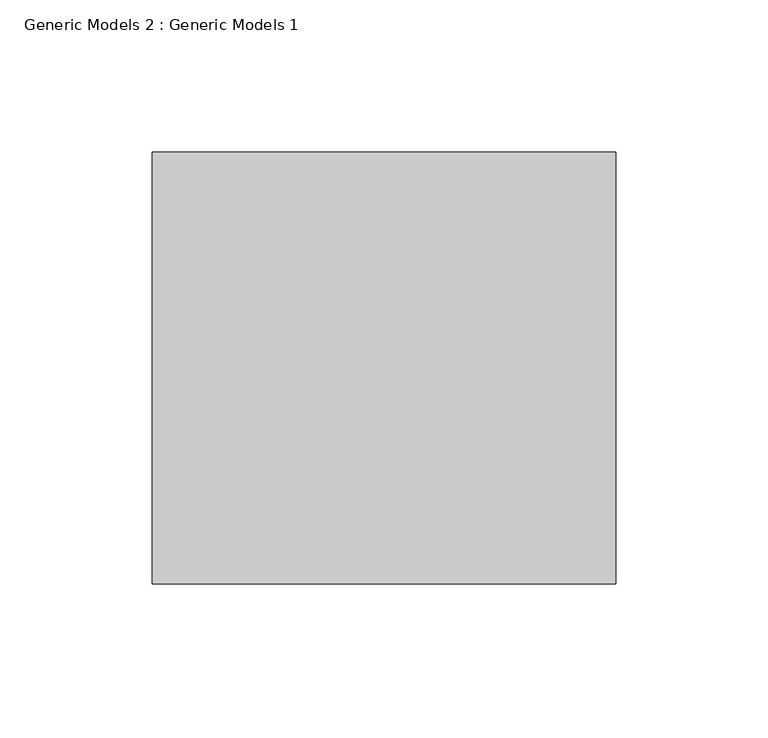
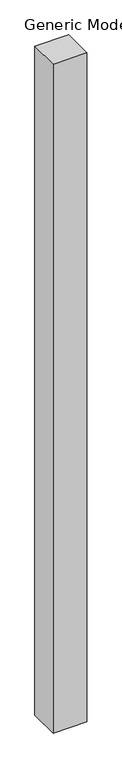
"""IFC4 building model written with IfcOpenShell, lengths in millimetres: proxy geometry, Generic Models 2 : Generic Models 1."""

from ifc_helpers import new_model, si_unit, origin, origin_with_axes, place, context, project, spatial, polyline, outline, extrude, source, transform, mapped, element, save


def generic_models_2_generic_models_1_277b538b(model_context):
    return source(origin(), model_context, "Body", "SweptSolid", [
        extrude(outline(polyline([(-12100.1536806, -5471.7273102), (-11947.7536806, -5471.7273102), (-11947.7536806, -5613.7098142), (-12100.1536806, -5613.7098142), (-12100.1536806, -5471.7273102)])), origin_with_axes(), (0.0, 0.0, 1.0), 3200.4),
    ])


if __name__ == "__main__":
    model = new_model("IFC4")
    model_context = context("Model", 3, world=origin())
    ifc_project = project(units=[si_unit("LENGTHUNIT", "METRE", prefix="MILLI")], contexts=[model_context])
    site = spatial("IfcSite", under=ifc_project)
    building = spatial("IfcBuilding", under=site)
    placement = place(None, origin())
    generic_models_2_generic_models_1_shape = generic_models_2_generic_models_1_277b538b(model_context)
    element("IfcBuildingElementProxy", 1, Name="Generic Models 2 : Generic Models 1", ObjectType="Generic Models 2 : Generic Models 1", at=placement, inside=building, context=model_context, shape_type="MappedRepresentation", body=[
        mapped(generic_models_2_generic_models_1_shape, transform((0.0, 0.0, 0.0), x_axis=(1.0, 0.0, 0.0), y_axis=(0.0, 1.0, 0.0), z_axis=(0.0, 0.0, 1.0))),
    ])
    save(model, "model.ifc")
